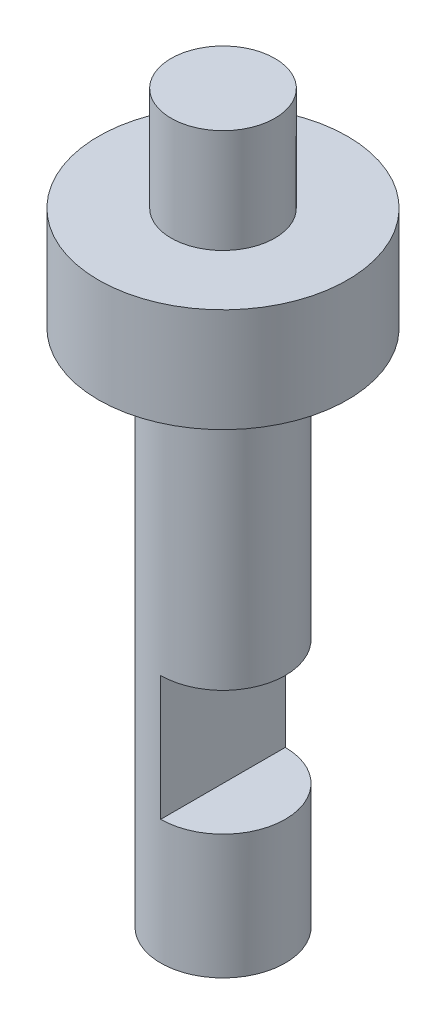
from build123d import *

# Parameters (mm, degrees)
SIDE_NOTCH_SKETCH_W  = 8.527366903
SIDE_NOTCH_SKETCH_H  = 6
SIDE_NOTCH_6X6_DEPTH = 9.5


with BuildPart() as part:
    # Pin Profile Sketch → Pin Body (revolve)
    with BuildSketch(Plane.XY, mode=Mode.PRIVATE) as pin_body_sk:
        Polygon((0, 0), (-2.5, 0), (-2.5, -5), (-6, -5), (-6, -10), (-3, -10), (-3, -35), (0, -35), align=None)
    revolve(pin_body_sk.sketch.rotate(Axis((0, -35, 0), (0, 1, 0)), 270), axis=Axis((0, -35, 0), (0, 1, 0)))

    # Side Notch Sketch → Side Notch 6x6 (cut, symmetric)
    with BuildSketch(Plane.XY):
        with Locations((4.263683452, -26)):
            Rectangle(SIDE_NOTCH_SKETCH_W, SIDE_NOTCH_SKETCH_H)
    extrude(amount=SIDE_NOTCH_6X6_DEPTH, both=True, mode=Mode.SUBTRACT)


solid = part.part
